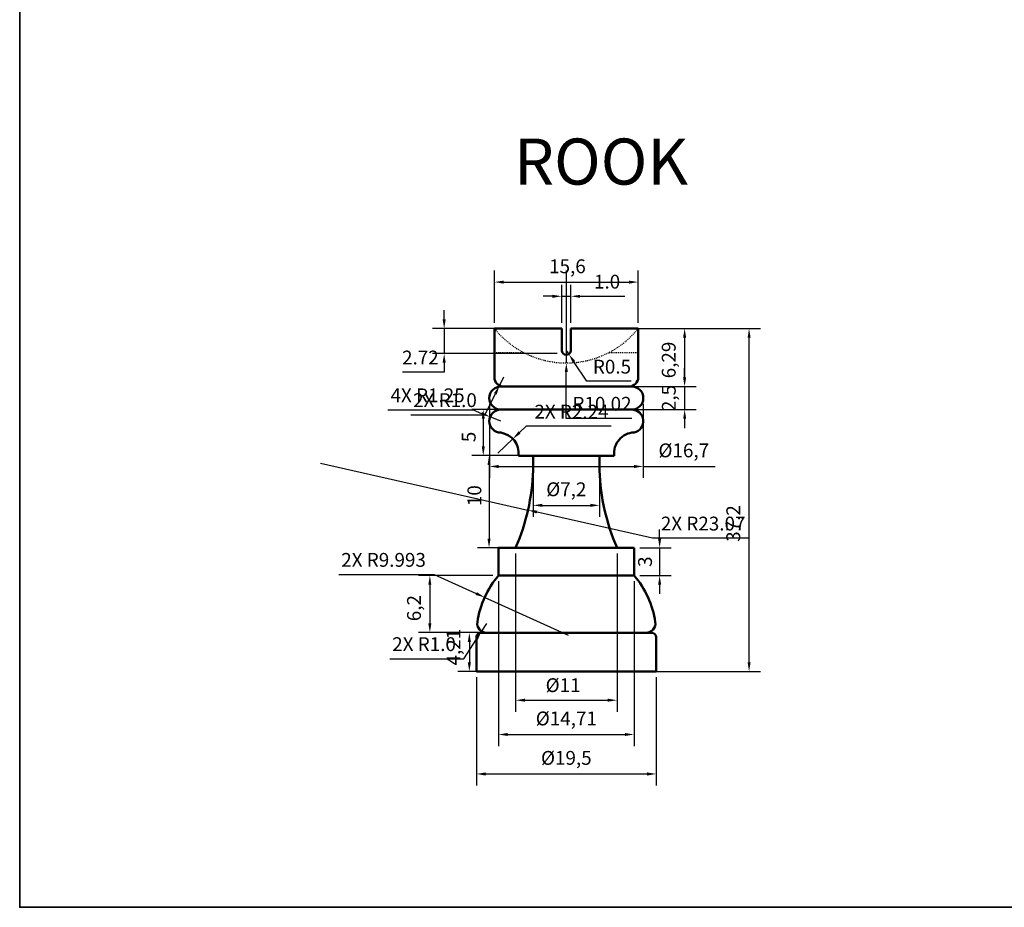
# Model space of a CAD drawing. Units: millimetres. Extents: x 172 to 469, y -14 to 196.
# Tile 1 of 5: x 172 to 279, y -14 to 82. Entities that reach past the tile are written whole.
import ezdxf

# ---------------------------------------------------------------- set-up
doc = ezdxf.new("R2010")
doc.units = ezdxf.units.MM
doc.header["$LTSCALE"] = 0.1
doc.linetypes.add('HIDDEN', pattern=[9.525, 6.35, -3.175])
for name, color, linetype, lineweight in [('M-DIMS', 2, 'Continuous', 25), ('M-HIDN', 1, 'HIDDEN', 25), ('M-OUTL', 7, 'Continuous', 50), ('M-TEXT', 3, 'Continuous', 25), ('M-TTLB', 7, 'Continuous', 35)]:
    doc.layers.add(name, color=color, linetype=linetype, lineweight=lineweight)
doc.styles.get("Standard").update_dxf_attribs({"font": 'arial.ttf'})
doc.dimstyles.new('ISO-25', dxfattribs={"dimtxt": 1.5, "dimasz": 1, "dimexe": 1.25, "dimexo": 0.625, "dimtad": 1, "dimtoh": 1, "dimtxsty": 'Standard', "dimcen": 2.5, "dimadec": 0, "dimazin": 0, "dimtfac": 1, "dimtmove": 0, "dimatfit": 3, "dimfxl": 1, "dimarcsym": 0})

# ---------------------------------------------------------------- blocks, each defined once
blk = doc.blocks.new('*D45')
at = {"layer": 'Defpoints', "color": 0, "ltscale": 0.1, "transparency": 16777216}
for p in [(239.48, 53.69), (223.88, 48.65), (239.48, 48.65)]:
    blk.add_point(p, dxfattribs=at)
at = {"layer": 'M-DIMS', "color": 0, "lineweight": -2, "ltscale": 0.1, "transparency": 16777216}
for p, q in [((223.88, 49.27), (223.88, 54.94)), ((239.48, 49.27), (239.48, 54.94)), ((224.88, 53.69), (238.48, 53.69))]:
    blk.add_line(p, q, dxfattribs=at)
at = {"layer": 'M-DIMS', "color": 0, "ltscale": 0.1, "transparency": 16777216}
for points in [[(224.88, 53.85), (224.88, 53.52), (223.88, 53.69)], [(238.48, 53.85), (238.48, 53.52), (239.48, 53.69)]]:
    blk.add_solid(points, dxfattribs=at)
at = {"layer": 'M-DIMS', "color": 0, "ltscale": 0.1, "transparency": 16777216, "insert": (231.8, 55.21), "char_height": 1.5, "attachment_point": 5}
blk.add_mtext('15,6', dxfattribs=at)
blk = doc.blocks.new('*D46')
at = {"layer": 'Defpoints', "color": 0, "ltscale": 0.1, "transparency": 16777216}
for p in [(237.77, 48.65), (237.77, 42.36), (244.51, 42.36)]:
    blk.add_point(p, dxfattribs=at)
at = {"layer": 'M-DIMS', "color": 0, "lineweight": -2, "ltscale": 0.1, "transparency": 16777216}
for p, q in [((238.4, 48.65), (245.76, 48.65)), ((244.51, 47.65), (244.51, 43.36)), ((238.4, 42.36), (245.76, 42.36))]:
    blk.add_line(p, q, dxfattribs=at)
at = {"layer": 'M-DIMS', "color": 0, "ltscale": 0.1, "transparency": 16777216}
for points in [[(244.34, 47.65), (244.68, 47.65), (244.51, 48.65)], [(244.34, 43.36), (244.68, 43.36), (244.51, 42.36)]]:
    blk.add_solid(points, dxfattribs=at)
at = {"layer": 'M-DIMS', "color": 0, "ltscale": 0.1, "transparency": 16777216, "insert": (242.98, 45.24), "char_height": 1.5, "attachment_point": 5, "rotation": 90}
blk.add_mtext('6,29', dxfattribs=at)
blk = doc.blocks.new('*D47')
at = {"layer": 'Defpoints', "color": 0, "ltscale": 0.1, "transparency": 16777216}
for p in [(237.77, 42.36), (237.77, 39.86), (244.51, 39.86)]:
    blk.add_point(p, dxfattribs=at)
at = {"layer": 'M-DIMS', "color": 0, "lineweight": -2, "ltscale": 0.1, "transparency": 16777216}
for p, q in [((244.51, 43.36), (244.51, 44.36)), ((238.4, 42.36), (245.76, 42.36)), ((244.51, 42.36), (244.51, 39.86)), ((238.4, 39.86), (245.76, 39.86)), ((244.51, 38.86), (244.51, 37.86))]:
    blk.add_line(p, q, dxfattribs=at)
at = {"layer": 'M-DIMS', "color": 0, "ltscale": 0.1, "transparency": 16777216}
for points in [[(244.35, 43.36), (244.68, 43.36), (244.51, 42.36)], [(244.35, 38.86), (244.68, 38.86), (244.51, 39.86)]]:
    blk.add_solid(points, dxfattribs=at)
at = {"layer": 'M-DIMS', "color": 0, "ltscale": 0.1, "transparency": 16777216, "insert": (242.99, 41.11), "char_height": 1.5, "attachment_point": 5, "rotation": 90}
blk.add_mtext('2,5', dxfattribs=at)
blk = doc.blocks.new('*D48')
at = {"layer": 'Defpoints', "color": 0, "ltscale": 0.1, "transparency": 16777216}
for p in [(231.68, 39.86), (222.67, 34.86), (231.68, 34.86)]:
    blk.add_point(p, dxfattribs=at)
at = {"layer": 'M-DIMS', "color": 0, "lineweight": -2, "ltscale": 0.1, "transparency": 16777216}
for p, q in [((231.05, 39.86), (221.42, 39.86)), ((222.67, 38.86), (222.67, 35.86)), ((231.05, 34.86), (221.42, 34.86))]:
    blk.add_line(p, q, dxfattribs=at)
at = {"layer": 'M-DIMS', "color": 0, "ltscale": 0.1, "transparency": 16777216}
for points in [[(222.51, 38.86), (222.84, 38.86), (222.67, 39.86)], [(222.51, 35.86), (222.84, 35.86), (222.67, 34.86)]]:
    blk.add_solid(points, dxfattribs=at)
at = {"layer": 'M-DIMS', "color": 0, "ltscale": 0.1, "transparency": 16777216, "insert": (221.29, 36.89), "char_height": 1.5, "attachment_point": 5, "rotation": 90}
blk.add_mtext('5', dxfattribs=at)
blk = doc.blocks.new('*D49')
at = {"layer": 'Defpoints', "color": 0, "ltscale": 0.1, "transparency": 16777216}
for p in [(223.33, 41.11), (240.03, 41.11), (240.03, 33.69)]:
    blk.add_point(p, dxfattribs=at)
at = {"layer": 'M-DIMS', "color": 0, "lineweight": -2, "ltscale": 0.1, "transparency": 16777216}
for p, q in [((223.33, 40.48), (223.33, 32.44)), ((240.03, 40.48), (240.03, 32.44)), ((224.33, 33.69), (239.03, 33.69)), ((240.03, 33.69), (247.81, 33.69))]:
    blk.add_line(p, q, dxfattribs=at)
at = {"layer": 'M-DIMS', "color": 0, "ltscale": 0.1, "transparency": 16777216}
for points in [[(224.33, 33.85), (224.33, 33.52), (223.33, 33.69)], [(239.03, 33.85), (239.03, 33.52), (240.03, 33.69)]]:
    blk.add_solid(points, dxfattribs=at)
at = {"layer": 'M-DIMS', "color": 0, "ltscale": 0.1, "transparency": 16777216, "insert": (244.42, 35.24), "char_height": 1.5, "attachment_point": 5}
blk.add_mtext('%%C16,7', dxfattribs=at)
blk = doc.blocks.new('*D50')
at = {"layer": 'Defpoints', "color": 0, "ltscale": 0.1, "transparency": 16777216}
for p in [(228.08, 34.86), (235.28, 34.86), (235.28, 29.47)]:
    blk.add_point(p, dxfattribs=at)
at = {"layer": 'M-DIMS', "color": 0, "lineweight": -2, "ltscale": 0.1, "transparency": 16777216}
for p, q in [((228.08, 34.23), (228.08, 28.22)), ((235.28, 34.23), (235.28, 28.22)), ((229.08, 29.47), (234.28, 29.47))]:
    blk.add_line(p, q, dxfattribs=at)
at = {"layer": 'M-DIMS', "color": 0, "ltscale": 0.1, "transparency": 16777216}
for points in [[(229.08, 29.64), (229.08, 29.3), (228.08, 29.47)], [(234.28, 29.64), (234.28, 29.3), (235.28, 29.47)]]:
    blk.add_solid(points, dxfattribs=at)
at = {"layer": 'M-DIMS', "color": 0, "ltscale": 0.1, "transparency": 16777216, "insert": (231.68, 31.02), "char_height": 1.5, "attachment_point": 5}
blk.add_mtext('%%C7,2', dxfattribs=at)
blk = doc.blocks.new('*D51')
at = {"layer": 'Defpoints', "color": 0, "ltscale": 0.1, "transparency": 16777216}
for p in [(239.03, 24.86), (239.03, 21.86), (241.8, 21.86)]:
    blk.add_point(p, dxfattribs=at)
at = {"layer": 'M-DIMS', "color": 0, "lineweight": -2, "ltscale": 0.1, "transparency": 16777216}
for p, q in [((241.8, 25.86), (241.8, 26.86)), ((239.66, 24.86), (243.05, 24.86)), ((241.8, 24.86), (241.8, 21.86)), ((239.66, 21.86), (243.05, 21.86)), ((241.8, 20.86), (241.8, 19.86))]:
    blk.add_line(p, q, dxfattribs=at)
at = {"layer": 'M-DIMS', "color": 0, "ltscale": 0.1, "transparency": 16777216}
for points in [[(241.63, 25.86), (241.97, 25.86), (241.8, 24.86)], [(241.63, 20.86), (241.97, 20.86), (241.8, 21.86)]]:
    blk.add_solid(points, dxfattribs=at)
at = {"layer": 'M-DIMS', "color": 0, "ltscale": 0.1, "transparency": 16777216, "insert": (240.41, 23.36), "char_height": 1.5, "attachment_point": 5, "rotation": 90}
blk.add_mtext('3', dxfattribs=at)
blk = doc.blocks.new('*D52')
at = {"layer": 'Defpoints', "color": 0, "ltscale": 0.1, "transparency": 16777216}
for p in [(224.32, 21.86), (216.88, 15.66), (224.32, 15.66)]:
    blk.add_point(p, dxfattribs=at)
at = {"layer": 'M-DIMS', "color": 0, "lineweight": -2, "ltscale": 0.1, "transparency": 16777216}
for p, q in [((223.7, 21.86), (215.63, 21.86)), ((216.88, 20.86), (216.88, 16.66)), ((223.7, 15.66), (215.63, 15.66))]:
    blk.add_line(p, q, dxfattribs=at)
at = {"layer": 'M-DIMS', "color": 0, "ltscale": 0.1, "transparency": 16777216}
for points in [[(216.71, 20.86), (217.04, 20.86), (216.88, 21.86)], [(216.71, 16.66), (217.04, 16.66), (216.88, 15.66)]]:
    blk.add_solid(points, dxfattribs=at)
at = {"layer": 'M-DIMS', "color": 0, "ltscale": 0.1, "transparency": 16777216, "insert": (215.35, 18.32), "char_height": 1.5, "attachment_point": 5, "rotation": 90}
blk.add_mtext('6,2', dxfattribs=at)
blk = doc.blocks.new('*D53')
at = {"layer": 'Defpoints', "color": 0, "ltscale": 0.1, "transparency": 16777216}
for p in [(224.32, 15.66), (221.16, 11.45), (224.32, 11.45)]:
    blk.add_point(p, dxfattribs=at)
at = {"layer": 'M-DIMS', "color": 0, "lineweight": -2, "ltscale": 0.1, "transparency": 16777216}
for p, q in [((223.7, 15.66), (219.91, 15.66)), ((221.16, 14.66), (221.16, 12.45)), ((223.7, 11.45), (219.91, 11.45))]:
    blk.add_line(p, q, dxfattribs=at)
at = {"layer": 'M-DIMS', "color": 0, "ltscale": 0.1, "transparency": 16777216}
for points in [[(220.99, 14.66), (221.33, 14.66), (221.16, 15.66)], [(220.99, 12.45), (221.33, 12.45), (221.16, 11.45)]]:
    blk.add_solid(points, dxfattribs=at)
at = {"layer": 'M-DIMS', "color": 0, "ltscale": 0.1, "transparency": 16777216, "insert": (219.63, 14.09), "char_height": 1.5, "attachment_point": 5, "rotation": 90}
blk.add_mtext('4,21', dxfattribs=at)
blk = doc.blocks.new('*D54')
at = {"layer": 'Defpoints', "color": 0, "ltscale": 0.1, "transparency": 16777216}
for p in [(221.93, 11.45), (241.43, 11.45), (241.43, 0.33)]:
    blk.add_point(p, dxfattribs=at)
at = {"layer": 'M-DIMS', "color": 0, "lineweight": -2, "ltscale": 0.1, "transparency": 16777216}
for p, q in [((221.93, 10.82), (221.93, -0.92)), ((241.43, 10.82), (241.43, -0.92)), ((222.93, 0.33), (240.43, 0.33))]:
    blk.add_line(p, q, dxfattribs=at)
at = {"layer": 'M-DIMS', "color": 0, "ltscale": 0.1, "transparency": 16777216}
for points in [[(222.93, 0.5), (222.93, 0.16), (221.93, 0.33)], [(240.43, 0.5), (240.43, 0.16), (241.43, 0.33)]]:
    blk.add_solid(points, dxfattribs=at)
at = {"layer": 'M-DIMS', "color": 0, "ltscale": 0.1, "transparency": 16777216, "insert": (231.68, 1.88), "char_height": 1.5, "attachment_point": 5}
blk.add_mtext('%%C19,5', dxfattribs=at)
blk = doc.blocks.new('*D55')
at = {"layer": 'Defpoints', "color": 0, "ltscale": 0.1, "transparency": 16777216}
for p in [(224.32, 21.86), (239.03, 21.86), (239.03, 4.61)]:
    blk.add_point(p, dxfattribs=at)
at = {"layer": 'M-DIMS', "color": 0, "lineweight": -2, "ltscale": 0.1, "transparency": 16777216}
for p, q in [((224.32, 21.23), (224.32, 3.36)), ((239.03, 21.23), (239.03, 3.36)), ((225.32, 4.61), (238.03, 4.61))]:
    blk.add_line(p, q, dxfattribs=at)
at = {"layer": 'M-DIMS', "color": 0, "ltscale": 0.1, "transparency": 16777216}
for points in [[(225.32, 4.78), (225.32, 4.45), (224.32, 4.61)], [(238.03, 4.78), (238.03, 4.45), (239.03, 4.61)]]:
    blk.add_solid(points, dxfattribs=at)
at = {"layer": 'M-DIMS', "color": 0, "ltscale": 0.1, "transparency": 16777216, "insert": (231.68, 6.16), "char_height": 1.5, "attachment_point": 5}
blk.add_mtext('%%C14,71', dxfattribs=at)
blk = doc.blocks.new('*D56')
at = {"layer": 'Defpoints', "color": 0, "ltscale": 0.1, "transparency": 16777216}
for p in [(226.18, 24.86), (237.18, 24.86), (237.18, 8.33)]:
    blk.add_point(p, dxfattribs=at)
at = {"layer": 'M-DIMS', "color": 0, "lineweight": -2, "ltscale": 0.1, "transparency": 16777216}
for p, q in [((226.18, 24.23), (226.18, 7.08)), ((237.18, 24.23), (237.18, 7.08)), ((227.18, 8.33), (236.18, 8.33))]:
    blk.add_line(p, q, dxfattribs=at)
at = {"layer": 'M-DIMS', "color": 0, "ltscale": 0.1, "transparency": 16777216}
for points in [[(227.18, 8.5), (227.18, 8.17), (226.18, 8.33)], [(236.18, 8.5), (236.18, 8.17), (237.18, 8.33)]]:
    blk.add_solid(points, dxfattribs=at)
at = {"layer": 'M-DIMS', "color": 0, "ltscale": 0.1, "transparency": 16777216, "insert": (231.33, 9.77), "char_height": 1.5, "attachment_point": 5}
blk.add_mtext('%%C11', dxfattribs=at)
blk = doc.blocks.new('*D57')
at = {"layer": 'Defpoints', "color": 0, "ltscale": 0.1, "transparency": 16777216}
for p in [(237.77, 48.65), (251.5, 48.65), (231.68, 11.45)]:
    blk.add_point(p, dxfattribs=at)
at = {"layer": 'M-DIMS', "color": 0, "lineweight": -2, "ltscale": 0.1, "transparency": 16777216}
for p, q in [((238.4, 48.65), (252.75, 48.65)), ((251.5, 12.45), (251.5, 47.65)), ((232.3, 11.45), (252.75, 11.45))]:
    blk.add_line(p, q, dxfattribs=at)
at = {"layer": 'M-DIMS', "color": 0, "ltscale": 0.1, "transparency": 16777216}
for points in [[(251.34, 47.65), (251.67, 47.65), (251.5, 48.65)], [(251.34, 12.45), (251.67, 12.45), (251.5, 11.45)]]:
    blk.add_solid(points, dxfattribs=at)
at = {"layer": 'M-DIMS', "color": 0, "ltscale": 0.1, "transparency": 16777216, "insert": (249.98, 27.5), "char_height": 1.5, "attachment_point": 5, "rotation": 90}
blk.add_mtext('37,2', dxfattribs=at)
blk = doc.blocks.new('*D58')
at = {"layer": 'Defpoints', "color": 0, "ltscale": 0.1, "transparency": 16777216}
for p in [(231.68, 34.86), (223.3, 24.86), (231.68, 24.86)]:
    blk.add_point(p, dxfattribs=at)
at = {"layer": 'M-DIMS', "color": 0, "lineweight": -2, "ltscale": 0.1, "transparency": 16777216}
for p, q in [((231.05, 34.86), (222.05, 34.86)), ((223.3, 33.86), (223.3, 25.86)), ((231.05, 24.86), (222.05, 24.86))]:
    blk.add_line(p, q, dxfattribs=at)
at = {"layer": 'M-DIMS', "color": 0, "ltscale": 0.1, "transparency": 16777216}
for points in [[(223.13, 33.86), (223.46, 33.86), (223.3, 34.86)], [(223.13, 25.86), (223.46, 25.86), (223.3, 24.86)]]:
    blk.add_solid(points, dxfattribs=at)
at = {"layer": 'M-DIMS', "color": 0, "ltscale": 0.1, "transparency": 16777216, "insert": (221.9, 30.52), "char_height": 1.5, "attachment_point": 5, "rotation": 90}
blk.add_mtext('10', dxfattribs=at)
blk = doc.blocks.new('*D64')
at = {"layer": 'Defpoints', "color": 0, "ltscale": 0.1, "transparency": 16777216}
for p in [(232.18, 52.15), (231.18, 48.65), (232.18, 48.65)]:
    blk.add_point(p, dxfattribs=at)
at = {"layer": 'M-DIMS', "color": 0, "lineweight": -2, "ltscale": 0.1, "transparency": 16777216}
for p, q in [((231.18, 49.27), (231.18, 53.4)), ((232.18, 49.27), (232.18, 53.4)), ((230.18, 52.15), (229.18, 52.15)), ((231.18, 52.15), (232.18, 52.15)), ((233.18, 52.15), (238.01, 52.15))]:
    blk.add_line(p, q, dxfattribs=at)
at = {"layer": 'M-DIMS', "color": 0, "ltscale": 0.1, "transparency": 16777216}
for points in [[(230.18, 52.31), (230.18, 51.98), (231.18, 52.15)], [(233.18, 52.31), (233.18, 51.98), (232.18, 52.15)]]:
    blk.add_solid(points, dxfattribs=at)
at = {"layer": 'M-DIMS', "color": 0, "ltscale": 0.1, "transparency": 16777216, "insert": (236.1, 53.54), "char_height": 1.5, "attachment_point": 5}
blk.add_mtext('1.0', dxfattribs=at)
blk = doc.blocks.new('*D65')
at = {"layer": 'Defpoints', "color": 0, "ltscale": 0.1, "transparency": 16777216}
for p in [(231.18, 48.65), (218.43, 45.93), (231.32, 45.93)]:
    blk.add_point(p, dxfattribs=at)
at = {"layer": 'M-DIMS', "color": 0, "lineweight": -2, "ltscale": 0.1, "transparency": 16777216}
for p, q in [((218.43, 49.65), (218.43, 50.65)), ((230.55, 48.65), (217.18, 48.65)), ((218.43, 48.65), (218.43, 45.93)), ((230.7, 45.93), (217.18, 45.93)), ((218.43, 44.93), (218.43, 43.93)), ((218.43, 43.93), (213.9, 43.93))]:
    blk.add_line(p, q, dxfattribs=at)
at = {"layer": 'M-DIMS', "color": 0, "ltscale": 0.1, "transparency": 16777216}
for points in [[(218.26, 49.65), (218.6, 49.65), (218.43, 48.65)], [(218.26, 44.93), (218.6, 44.93), (218.43, 45.93)]]:
    blk.add_solid(points, dxfattribs=at)
at = {"layer": 'M-DIMS', "color": 0, "ltscale": 0.1, "transparency": 16777216, "insert": (215.85, 45.31), "char_height": 1.5, "attachment_point": 5}
blk.add_mtext('2.72', dxfattribs=at)
blk = doc.blocks.new('*D88')
at = {"layer": 'Defpoints', "color": 0, "ltscale": 0.1, "transparency": 16777216}
for p in [(205.02, 34.06), (227.52, 28.96)]:
    blk.add_point(p, dxfattribs=at)
at = {"layer": 'M-DIMS', "color": 0, "lineweight": -2, "ltscale": 0.1, "transparency": 16777216}
for p, q in [((205.02, 34.06), (227.52, 28.96)), ((241.02, 25.91), (228.5, 28.74)), ((251.39, 25.91), (241.02, 25.91))]:
    blk.add_line(p, q, dxfattribs=at)
at = {"layer": 'M-DIMS', "color": 0, "ltscale": 0.1, "transparency": 16777216}
blk.add_solid([(228.53, 28.9), (228.46, 28.58), (227.52, 28.96)], dxfattribs=at)
at = {"layer": 'M-DIMS', "color": 0, "ltscale": 0.1, "transparency": 16777216, "insert": (246.52, 27.3), "char_height": 1.5, "attachment_point": 5}
blk.add_mtext('2X R23.07', dxfattribs=at)
blk = doc.blocks.new('*D89')
at = {"layer": 'Defpoints', "color": 0, "ltscale": 0.1, "transparency": 16777216}
for p in [(231.68, 54.94), (231.68, 44.92)]:
    blk.add_point(p, dxfattribs=at)
at = {"layer": 'M-DIMS', "color": 0, "lineweight": -2, "ltscale": 0.1, "transparency": 16777216}
for p, q in [((231.68, 54.94), (231.68, 44.92)), ((231.68, 38.9), (231.68, 43.92)), ((238.79, 38.9), (231.68, 38.9))]:
    blk.add_line(p, q, dxfattribs=at)
at = {"layer": 'M-DIMS', "color": 0, "ltscale": 0.1, "transparency": 16777216}
blk.add_solid([(231.85, 43.92), (231.51, 43.92), (231.68, 44.92)], dxfattribs=at)
at = {"layer": 'M-DIMS', "color": 0, "ltscale": 0.1, "transparency": 16777216, "insert": (235.55, 40.29), "char_height": 1.5, "attachment_point": 5}
blk.add_mtext('R10.02', dxfattribs=at)
blk = doc.blocks.new('*D90')
at = {"layer": 'Defpoints', "color": 0, "ltscale": 0.1, "transparency": 16777216}
for p in [(222.82, 19.49), (231.92, 15.36)]:
    blk.add_point(p, dxfattribs=at)
at = {"layer": 'M-DIMS', "color": 0, "lineweight": -2, "ltscale": 0.1, "transparency": 16777216}
for p, q in [((206.99, 21.97), (217.36, 21.97)), ((217.36, 21.97), (221.91, 19.9)), ((231.92, 15.36), (222.82, 19.49))]:
    blk.add_line(p, q, dxfattribs=at)
at = {"layer": 'M-DIMS', "color": 0, "ltscale": 0.1, "transparency": 16777216}
blk.add_solid([(221.98, 20.06), (221.84, 19.75), (222.82, 19.49)], dxfattribs=at)
at = {"layer": 'M-DIMS', "color": 0, "ltscale": 0.1, "transparency": 16777216, "insert": (211.86, 23.36), "char_height": 1.5, "attachment_point": 5}
blk.add_mtext('2X R9.993', dxfattribs=at)
blk = doc.blocks.new('*D91')
at = {"layer": 'Defpoints', "color": 0, "ltscale": 0.1, "transparency": 16777216}
for p in [(225.88, 36.68), (224.25, 35.14)]:
    blk.add_point(p, dxfattribs=at)
at = {"layer": 'M-DIMS', "color": 0, "lineweight": -2, "ltscale": 0.1, "transparency": 16777216}
for p, q in [((227.33, 38.06), (226.6, 37.37)), ((236.53, 38.06), (227.33, 38.06)), ((224.25, 35.14), (225.88, 36.68))]:
    blk.add_line(p, q, dxfattribs=at)
at = {"layer": 'M-DIMS', "color": 0, "ltscale": 0.1, "transparency": 16777216}
blk.add_solid([(226.49, 37.49), (226.72, 37.25), (225.88, 36.68)], dxfattribs=at)
at = {"layer": 'M-DIMS', "color": 0, "ltscale": 0.1, "transparency": 16777216, "insert": (232.24, 39.44), "char_height": 1.5, "attachment_point": 5}
blk.add_mtext('2X R2.24', dxfattribs=at)
blk = doc.blocks.new('*D92')
at = {"layer": 'Defpoints', "color": 0, "ltscale": 0.1, "transparency": 16777216}
for p in [(223.42, 39.07), (224.58, 38.61)]:
    blk.add_point(p, dxfattribs=at)
at = {"layer": 'M-DIMS', "color": 0, "lineweight": -2, "ltscale": 0.1, "transparency": 16777216}
for p, q in [((212.31, 39.82), (221.56, 39.82)), ((221.56, 39.82), (222.49, 39.45)), ((224.58, 38.61), (223.42, 39.07))]:
    blk.add_line(p, q, dxfattribs=at)
at = {"layer": 'M-DIMS', "color": 0, "ltscale": 0.1, "transparency": 16777216}
blk.add_solid([(222.55, 39.6), (222.43, 39.29), (223.42, 39.07)], dxfattribs=at)
at = {"layer": 'M-DIMS', "color": 0, "ltscale": 0.1, "transparency": 16777216, "insert": (216.63, 41.21), "char_height": 1.5, "attachment_point": 5}
blk.add_mtext('4X R1.25', dxfattribs=at)
blk = doc.blocks.new('*D93')
at = {"layer": 'Defpoints', "color": 0, "ltscale": 0.1, "transparency": 16777216}
for p in [(224.88, 43.36), (224.43, 42.46)]:
    blk.add_point(p, dxfattribs=at)
at = {"layer": 'M-DIMS', "color": 0, "lineweight": -2, "ltscale": 0.1, "transparency": 16777216}
for p, q in [((224.88, 43.36), (224.43, 42.46)), ((222.85, 39.3), (223.98, 41.57)), ((214.82, 39.3), (222.85, 39.3))]:
    blk.add_line(p, q, dxfattribs=at)
at = {"layer": 'M-DIMS', "color": 0, "ltscale": 0.1, "transparency": 16777216}
blk.add_solid([(223.83, 41.64), (224.13, 41.49), (224.43, 42.46)], dxfattribs=at)
at = {"layer": 'M-DIMS', "color": 0, "ltscale": 0.1, "transparency": 16777216, "insert": (218.52, 40.69), "char_height": 1.5, "attachment_point": 5}
blk.add_mtext('2X R1.0', dxfattribs=at)
blk = doc.blocks.new('*D94')
at = {"layer": 'Defpoints', "color": 0, "ltscale": 0.1, "transparency": 16777216}
for p in [(223.02, 16.66), (222.48, 15.81)]:
    blk.add_point(p, dxfattribs=at)
at = {"layer": 'M-DIMS', "color": 0, "lineweight": -2, "ltscale": 0.1, "transparency": 16777216}
for p, q in [((223.02, 16.66), (222.48, 15.81)), ((220.58, 12.83), (221.94, 14.97)), ((212.55, 12.83), (220.58, 12.83))]:
    blk.add_line(p, q, dxfattribs=at)
at = {"layer": 'M-DIMS', "color": 0, "ltscale": 0.1, "transparency": 16777216}
blk.add_solid([(221.8, 15.06), (222.08, 14.88), (222.48, 15.81)], dxfattribs=at)
at = {"layer": 'M-DIMS', "color": 0, "ltscale": 0.1, "transparency": 16777216, "insert": (216.25, 14.22), "char_height": 1.5, "attachment_point": 5}
blk.add_mtext('2X R1.0', dxfattribs=at)
blk = doc.blocks.new('*D95')
at = {"layer": 'Defpoints', "color": 0, "ltscale": 0.1, "transparency": 16777216}
for p in [(231.68, 46.28), (231.96, 45.87)]:
    blk.add_point(p, dxfattribs=at)
at = {"layer": 'M-DIMS', "color": 0, "lineweight": -2, "ltscale": 0.1, "transparency": 16777216}
for p, q in [((231.68, 46.28), (231.96, 45.87)), ((233.92, 42.93), (232.51, 45.03)), ((238.72, 42.93), (233.92, 42.93))]:
    blk.add_line(p, q, dxfattribs=at)
at = {"layer": 'M-DIMS', "color": 0, "ltscale": 0.1, "transparency": 16777216}
blk.add_solid([(232.65, 45.13), (232.37, 44.94), (231.96, 45.87)], dxfattribs=at)
at = {"layer": 'M-DIMS', "color": 0, "ltscale": 0.1, "transparency": 16777216, "insert": (236.63, 44.32), "char_height": 1.5, "attachment_point": 5}
blk.add_mtext('R0.5', dxfattribs=at)

msp = doc.modelspace()

# ---------------------------------------------------------------- linework, layer by layer
at = {"layer": 'M-HIDN', "ltscale": 0.1}
for p, q in [((223.8785, 46.0468), (227.0547, 46.0468)), ((236.3024, 46.0468), (239.4785, 46.0468))]:
    msp.add_line(p, q, dxfattribs=at)
msp.add_arc((231.6785, 54.9364), 10.0202, 218.883061, 321.116939, dxfattribs=at)
at = {"layer": 'M-OUTL', "ltscale": 0.1}
for p, q in [((231.1785, 48.6464), (223.8785, 48.6464)), ((231.1785, 46.2813), (231.1785, 48.6464)), ((232.1785, 48.6464), (239.4785, 48.6464)), ((232.1785, 46.2813), (232.1785, 48.6464)), ((231.1785, 44.9162), (231.1785, 44.9287)), ((232.1785, 44.9162), (232.1785, 44.9287)), ((228.0785, 39.8564), (235.2785, 39.8564)), ((236.8785, 34.8564), (226.4785, 34.8564)), ((228.0785, 33.2567), (228.0785, 34.8564)), ((228.0785, 34.8564), (235.2785, 34.8564)), ((235.2785, 33.2567), (235.2785, 34.8564)), ((239.0335, 24.8564), (224.3235, 24.8564)), ((224.3235, 24.8564), (224.3235, 21.8564)), ((239.0335, 24.8564), (239.0335, 21.8564)), ((239.0335, 21.8564), (224.3235, 21.8564)), ((221.9285, 15.2032), (221.9285, 11.4464)), ((240.9285, 15.6564), (222.4263, 15.6564)), ((241.4285, 11.4464), (241.4285, 15.1564)), ((221.9285, 11.4464), (241.4285, 11.4464))]:
    msp.add_line(p, q, dxfattribs=at)
for points in [[(239.4785, 48.6464), (239.4785, 43.3564, -0.41421356), (238.4785, 42.3564), (224.8785, 42.3564, -0.41421356), (223.8785, 43.3564), (223.8785, 48.6464)], [(239.0251, 37.381, 0.90533942), (238.7785, 39.8564), (224.5785, 39.8564, 1), (224.5785, 37.3564), (224.593, 37.3564)]]:
    msp.add_lwpolyline(points, format="xyb", dxfattribs=at)
msp.add_lwpolyline([(238.7785, 42.3564), (224.5785, 42.3564, 1), (224.5785, 39.8564), (238.7785, 39.8564, 1)], format="xyb", close=True, dxfattribs=at)
for points in [[(224.5785, 39.8564), (238.7785, 39.8564)], [(238.7641, 37.3564), (238.7785, 37.3564)]]:
    msp.add_lwpolyline(points, dxfattribs=at)
for centre, radius, start, end in [((231.6785, 46.2813), 0.5, 180, 0), ((239.1044, 35.1387), 2.2437, 92.024705, 187.227787), ((224.2527, 35.1387), 2.2437, 352.772213, 81.275364), ((205.0225, 34.0565), 23.0699, 336.49715, 358.013084), ((258.3345, 34.0565), 23.0699, 181.986916, 203.50285), ((231.9176, 15.3603), 9.9935, 139.455816, 171.713875), ((231.4394, 15.3603), 9.9935, 8.286125, 40.544184), ((223.018, 16.6564), 1, 171.713875, 270), ((240.339, 16.6564), 1, 270, 8.286125), ((222.4263, 15.1564), 0.5, 90, 174.625393), ((240.9285, 15.1564), 0.5, 0, 90)]:
    msp.add_arc(centre, radius, start, end, dxfattribs=at)
at = {"layer": 'M-TTLB', "ltscale": 0.1}
msp.add_lwpolyline([(172.3921, 195.8665), (469.3921, 195.8665), (469.3921, -14.1335), (172.3921, -14.1335)], close=True, dxfattribs=at)

# ---------------------------------------------------------------- texts
at = {"layer": 'M-TEXT', "ltscale": 0.1, "insert": (213.3465, 69.2598), "char_height": 5, "attachment_point": 1}
msp.add_mtext_dynamic_manual_height_columns('\\pxqc;ROOK', width=44.206943, gutter_width=12.5, heights=[0], dxfattribs=at)

# ---------------------------------------------------------------- dimensions: what is measured, and where the dimension line sits
at = {"layer": 'M-DIMS', "ltscale": 0.1}
dim = msp.add_linear_dim(base=(239.4785, 53.6883), p1=(223.8785, 48.6464), p2=(239.4785, 48.6464), dimstyle='ISO-25', override={"dimclrd": 0, "dimclre": 0, "dimclrt": 0}, dxfattribs=at)
dim.commit()
dim.dimension.update_dxf_attribs({"geometry": '*D45', "text_midpoint": (231.7968, 53.6883), "dimtype": 160})
dim = msp.add_linear_dim(base=(232.1785, 52.1464), p1=(231.1785, 48.6464), p2=(232.1785, 48.6464), dimstyle='ISO-25', override={"dimdec": 1, "dimlfac": 1, "dimrnd": 0, "dimzin": 0, "dimdsep": 46, "dimlunit": 2}, dxfattribs=at)
dim.commit()
dim.dimension.update_dxf_attribs({"geometry": '*D64', "text_midpoint": (236.0958, 53.5373)})
dim = msp.add_radius_dim(center=(231.6785, 54.9364), mpoint=(231.679, 44.9162), dimstyle='ISO-25', override={"dimdec": 2, "dimlfac": 1, "dimrnd": 0, "dimzin": 0, "dimdsep": 46, "dimlunit": 2}, dxfattribs=at)
dim.commit()
dim.dimension.update_dxf_attribs({"geometry": '*D89', "text_midpoint": (235.5452, 38.9041), "dimtype": 164})
dim = msp.add_linear_dim(base=(218.4285, 45.9278), p1=(231.1785, 48.6464), p2=(231.325, 45.9278), angle=90, dimstyle='ISO-25', override={"dimdec": 2, "dimlfac": 1, "dimrnd": 0, "dimzin": 0, "dimdsep": 46, "dimlunit": 2}, dxfattribs=at)
dim.commit()
dim.dimension.update_dxf_attribs({"geometry": '*D65', "text_midpoint": (215.8503, 45.3058)})
for base, p1, p2, picture, middle in [((251.504, 48.6464), (231.6785, 11.4464), (237.7714, 48.6464), '*D57', (251.504, 27.4956)), ((244.5112, 42.3564), (237.7714, 48.6464), (237.7714, 42.3564), '*D46', (244.5112, 45.2398)), ((244.512, 39.8564), (237.7714, 42.3564), (237.7714, 39.8564), '*D47', (244.512, 41.1064)), ((222.6745, 34.8564), (231.6785, 39.8564), (231.6785, 34.8564), '*D48', (222.6745, 36.8893)), ((223.2957, 24.8564), (231.6785, 34.8564), (231.6785, 24.8564), '*D58', (223.2957, 30.5237)), ((241.7993, 21.8564), (239.0335, 24.8564), (239.0335, 21.8564), '*D51', (241.7993, 23.3564)), ((216.8768, 15.6564), (224.3235, 21.8564), (224.3235, 15.6564), '*D52', (216.8768, 18.3183)), ((221.1602, 11.4464), (224.3235, 15.6564), (224.3235, 11.4464), '*D53', (221.1602, 14.0932))]:
    dim = msp.add_linear_dim(base=base, p1=p1, p2=p2, angle=90, dimstyle='ISO-25', override={"dimclrd": 0, "dimclre": 0, "dimclrt": 0}, dxfattribs=at)
    dim.commit()
    dim.dimension.update_dxf_attribs({"geometry": picture, "text_midpoint": middle, "dimtype": 160})
dim = msp.add_radius_dim(center=(231.6785, 46.2813), mpoint=(231.9562, 45.8655), dimstyle='ISO-25', override={"dimdec": 1, "dimlfac": 1, "dimrnd": 0, "dimzin": 0, "dimdsep": 46, "dimlunit": 2}, dxfattribs=at)
dim.commit()
dim.dimension.update_dxf_attribs({"geometry": '*D95', "text_midpoint": (236.6316, 44.3195)})
for center, mpoint, text, override, picture, middle in [((224.5785, 38.6064), (223.4188, 39.0729), '4X <>', {"dimdec": 2, "dimlfac": 1, "dimrnd": 0, "dimzin": 0, "dimdsep": 46, "dimlunit": 2}, '*D92', (216.625, 41.2101)), ((224.8785, 43.3564), (224.431, 42.4621), '2X <>', {"dimdec": 1, "dimlfac": 1, "dimrnd": 0, "dimzin": 0, "dimdsep": 46, "dimlunit": 2}, '*D93', (218.5205, 40.6947)), ((224.2527, 35.1387), (225.8787, 36.6847), '2X <>', {"dimdec": 2, "dimlfac": 1, "dimrnd": 0, "dimzin": 0, "dimdsep": 46, "dimlunit": 2}, '*D91', (232.2403, 39.4414)), ((223.018, 16.6564), (222.4809, 15.8129), '2X <>', {"dimdec": 1, "dimlfac": 1, "dimrnd": 0, "dimzin": 0, "dimdsep": 46, "dimlunit": 2}, '*D94', (216.2537, 14.2249))]:
    dim = msp.add_radius_dim(center=center, mpoint=mpoint, text=text, dimstyle='ISO-25', override=override, dxfattribs=at)
    dim.commit()
    dim.dimension.update_dxf_attribs({"geometry": picture, "text_midpoint": middle})
for base, p1, p2, picture, middle in [((240.0285, 33.6881), (223.3285, 41.1064), (240.0285, 41.1064), '*D49', (244.4177, 33.6881)), ((235.2785, 29.4694), (228.0785, 34.8564), (235.2785, 34.8564), '*D50', (231.6785, 29.4694)), ((237.1785, 8.3341), (226.1785, 24.8564), (237.1785, 24.8564), '*D56', (231.3341, 8.3341)), ((239.0335, 4.6138), (224.3235, 21.8564), (239.0335, 21.8564), '*D55', (231.6785, 4.6138)), ((241.4285, 0.3304), (221.9285, 11.4464), (241.4285, 11.4464), '*D54', (231.6785, 0.3304))]:
    dim = msp.add_linear_dim(base=base, p1=p1, p2=p2, text='%%C<>', dimstyle='ISO-25', override={"dimclrd": 0, "dimclre": 0, "dimclrt": 0}, dxfattribs=at)
    dim.commit()
    dim.dimension.update_dxf_attribs({"geometry": picture, "text_midpoint": middle, "dimtype": 160})
for center, mpoint, override, picture, middle in [((205.0225, 34.0565), (227.5228, 28.9618), {"dimdec": 2, "dimlfac": 1, "dimrnd": 0, "dimzin": 0, "dimdsep": 46, "dimlunit": 2}, '*D88', (241.023, 25.905)), ((231.9176, 15.3603), (222.8178, 19.4911), {"dimdec": 3, "dimlfac": 1, "dimrnd": 0, "dimzin": 0, "dimdsep": 46, "dimlunit": 2}, '*D90', (211.86, 21.9695))]:
    dim = msp.add_radius_dim(center=center, mpoint=mpoint, text='2X <>', dimstyle='ISO-25', override=override, dxfattribs=at)
    dim.commit()
    dim.dimension.update_dxf_attribs({"geometry": picture, "text_midpoint": middle, "dimtype": 164})

doc.saveas('drawing.dxf')
